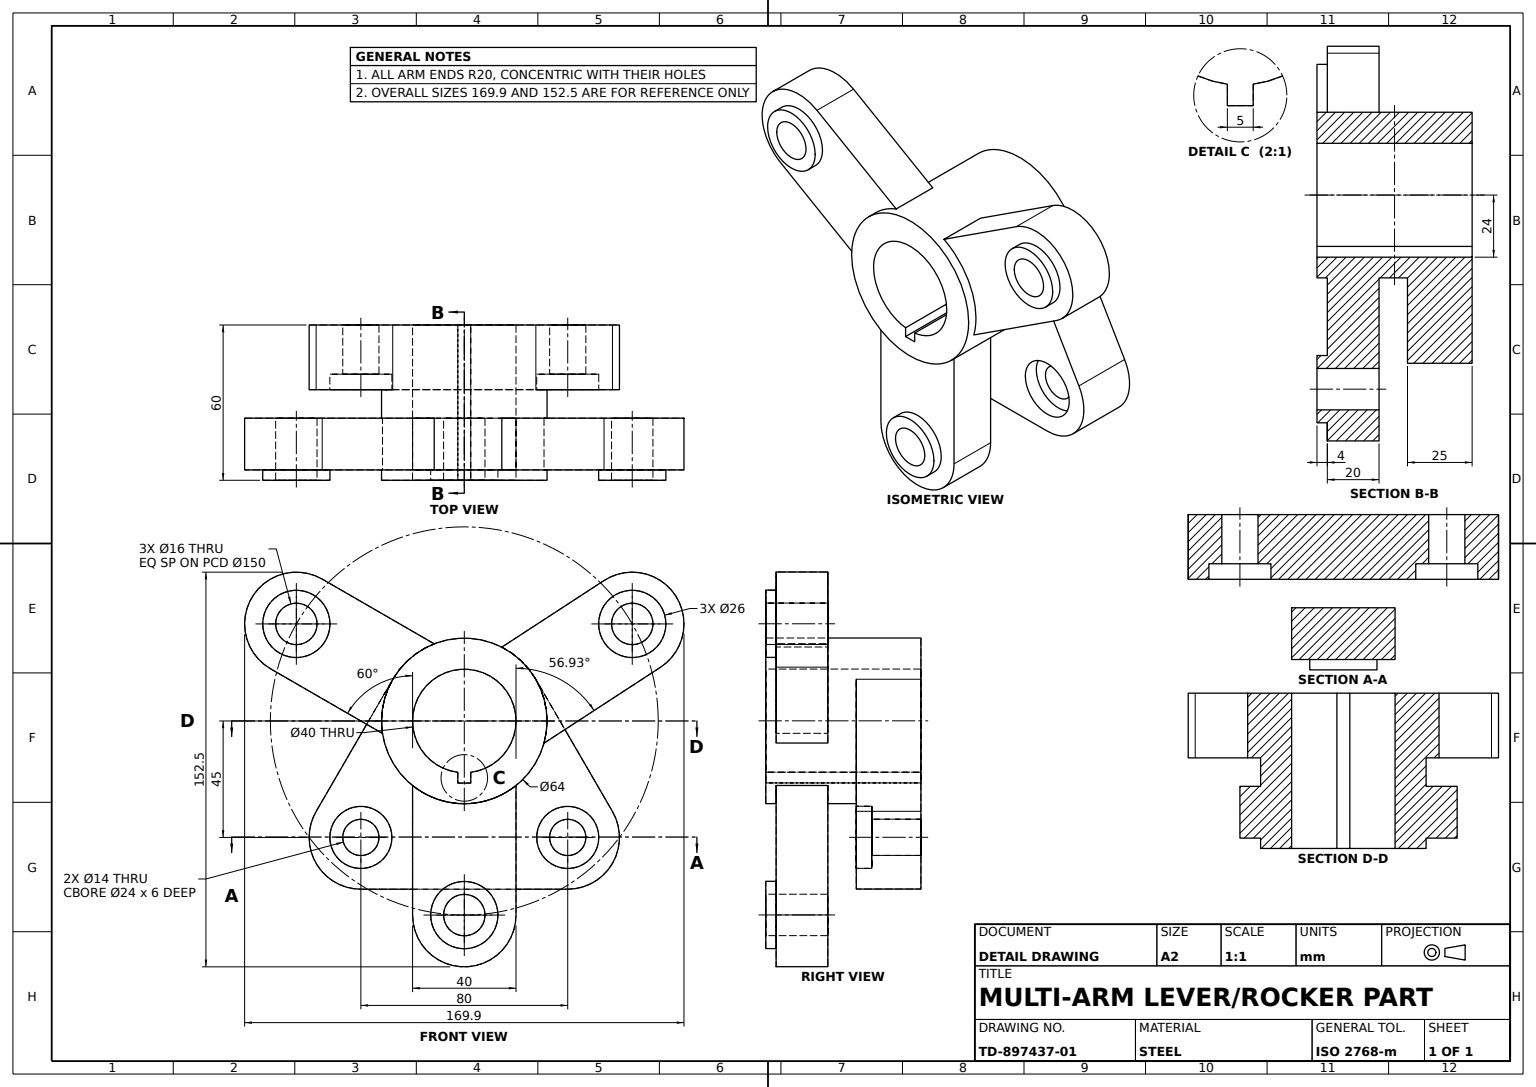
from build123d import *

# Parameters (mm, degrees)
LOWER_ARMS_25MM_DEPTH                 = 25
HUB_BOSS_SKETCH_32_R                  = 32
HUB_BOSS_32_DEPTH                     = 31
UPPER_START                           = -20
UPPER_ARMS_20MM_DEPTH                 = 20
HUB_COLLAR_SKETCH_32_R                = 32
HUB_COLLAR_32X4_DEPTH                 = 4
KEYED_HUB_BORE_DEPTH                  = 70
UPPER_ARM_PADS_SKETCH_3X_13_R         = 13
UPPER_ARM_PADS_3X_13_DEPTH            = 4
UPPER_ARM_HOLES_SKETCH_3X_8_R         = 8
UPPER_ARM_HOLES_3X_8_DEPTH            = 30
LOWER_ARM_COUNTERBORES_SKETCH_2X_12_R = 12
LOWER_ARM_COUNTERBORES_2X_12_DEPTH    = 6
LOWER_ARM_HOLES_SKETCH_2X_7_R         = 7
LOWER_ARM_HOLES_2X_7_DEPTH            = 20


with BuildPart() as part:
    # Lower Arms Profile → Lower Arms 25mm (new body)
    with BuildSketch(Plane.XY):
        with BuildLine():
            Line((-57.296551724, -34.95862069), (-27.674482759, 16.066206897))
            ThreePointArc((-27.674482759, 16.066206897), (0, 32), (27.674482759, 16.066206897))
            Line((27.674482759, 16.066206897), (57.296551724, -34.95862069))
            ThreePointArc((57.296551724, -34.95862069), (57.332449137, -54.979288897), (40, -65))
            Line((40, -65), (-40, -65))
            ThreePointArc((-40, -65), (-57.332449137, -54.979288897), (-57.296551724, -34.95862069))
        make_face()
    extrude(amount=LOWER_ARMS_25MM_DEPTH)

    # Hub Boss Sketch Ø32 → Hub Boss Ø32 (add)
    with BuildSketch(Plane.XY.offset(25)):
        with Locations(Location((0, 0, 0), (0, 0, 149.863023681))):
            Circle(HUB_BOSS_SKETCH_32_R)
    extrude(amount=HUB_BOSS_32_DEPTH)

    # Upper Arms Profile → Upper Arms 20mm (add)
    with BuildSketch(Plane.XY.offset(56).offset(UPPER_START)):
        with BuildLine():
            Line((-20, -24.979991994), (-20, -75))
            ThreePointArc((-20, -75), (0, -95), (20, -75))
            Line((20, -75), (20, -24.979991994))
            ThreePointArc((20, -24.979991994), (0, -32), (-20, -24.979991994))
        make_face()
        with BuildLine():
            ThreePointArc((-54.951905284, 54.820508076), (-82.27241336, 47.5), (-74.951905284, 20.179491924))
            Line((-74.951905284, 20.179491924), (-31.633307653, -4.830512079))
            ThreePointArc((-31.633307653, -4.830512079), (-27.712812921, 16), (-11.633307653, 29.810504072))
            Line((-11.633307653, 29.810504072), (-54.951905284, 54.820508076))
        make_face()
        with BuildLine():
            ThreePointArc((75.864190859, 20.73927139), (81.712633894, 48.412285575), (54.039619709, 54.26072861))
            Line((54.039619709, 54.26072861), (14.507199018, 28.522643227))
            ThreePointArc((14.507199018, 28.522643227), (29.291756215, 12.883827763), (30.827638328, -8.582349045))
            Line((30.827638328, -8.582349045), (75.864190859, 20.73927139))
        make_face()
    extrude(amount=UPPER_ARMS_20MM_DEPTH)

    # Hub Collar Sketch Ø32 → Hub Collar Ø32x4 (add)
    with BuildSketch(Plane.XY.offset(56)):
        with Locations(Location((0, 0, 0), (0, 0, 149.863023681))):
            Circle(HUB_COLLAR_SKETCH_32_R)
    extrude(amount=HUB_COLLAR_32X4_DEPTH)

    # Keyed Bore Sketch → Keyed Hub Bore (cut)
    with BuildSketch(Plane.XY.offset(60)):
        with BuildLine():
            Line((-2.5, -24), (2.5, -24))
            Line((2.5, -24), (2.5, -19.843134833))
            ThreePointArc((2.5, -19.843134833), (0, 20), (-2.5, -19.843134833))
            Line((-2.5, -19.843134833), (-2.5, -24))
        make_face()
    extrude(amount=-KEYED_HUB_BORE_DEPTH, mode=Mode.SUBTRACT)

    # Upper Arm Pads Sketch 3xØ13 → Upper Arm Pads 3xØ13 (add)
    with BuildSketch(Plane.XY.offset(56)):
        with Locations((-64.951905284, 37.5)):
            Circle(UPPER_ARM_PADS_SKETCH_3X_13_R)
        with Locations((64.951905284, 37.5)):
            Circle(UPPER_ARM_PADS_SKETCH_3X_13_R)
        with Locations((0, -75)):
            Circle(UPPER_ARM_PADS_SKETCH_3X_13_R)
    extrude(amount=UPPER_ARM_PADS_3X_13_DEPTH)

    # Upper Arm Holes Sketch 3xØ8 → Upper Arm Holes 3xØ8 (cut)
    with BuildSketch(Plane.XY.offset(60)):
        with Locations((-64.951905284, 37.5)):
            Circle(UPPER_ARM_HOLES_SKETCH_3X_8_R)
        with Locations((64.951905284, 37.5)):
            Circle(UPPER_ARM_HOLES_SKETCH_3X_8_R)
        with Locations((0, -75)):
            Circle(UPPER_ARM_HOLES_SKETCH_3X_8_R)
    extrude(amount=-UPPER_ARM_HOLES_3X_8_DEPTH, mode=Mode.SUBTRACT)

    # Lower Arm Counterbores Sketch 2xØ12 → Lower Arm Counterbores 2xØ12 (cut)
    with BuildSketch(Plane.XY.offset(25)):
        with Locations((-40, -45)):
            Circle(LOWER_ARM_COUNTERBORES_SKETCH_2X_12_R)
        with Locations((40, -45)):
            Circle(LOWER_ARM_COUNTERBORES_SKETCH_2X_12_R)
    extrude(amount=-LOWER_ARM_COUNTERBORES_2X_12_DEPTH, mode=Mode.SUBTRACT)

    # Lower Arm Holes Sketch 2xØ7 → Lower Arm Holes 2xØ7 (cut)
    with BuildSketch(Plane.XY.offset(19)):
        with Locations((-40, -45)):
            Circle(LOWER_ARM_HOLES_SKETCH_2X_7_R)
        with Locations((40, -45)):
            Circle(LOWER_ARM_HOLES_SKETCH_2X_7_R)
    extrude(amount=-LOWER_ARM_HOLES_2X_7_DEPTH, mode=Mode.SUBTRACT)


solid = part.part
